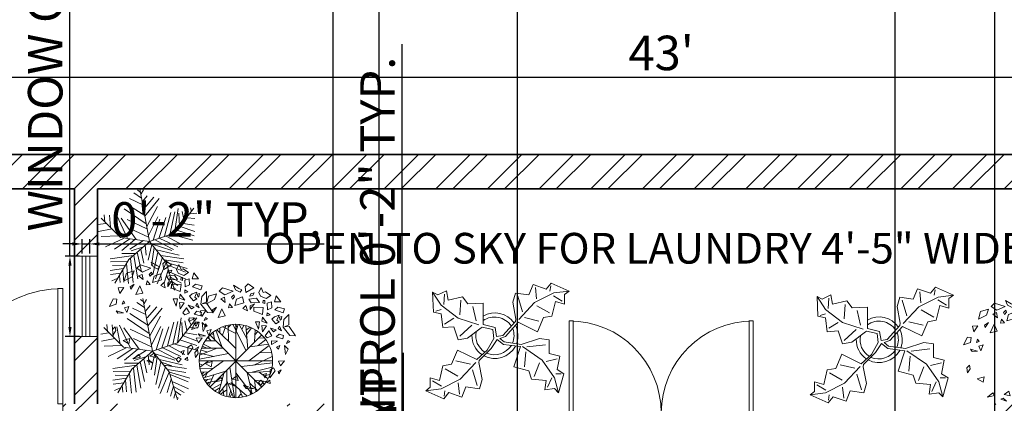
# Model space of a CAD drawing. Units: inches. Extents: x 744 to 1448, y 5126 to 6077.
# Tile 8 of 10: x 895 to 1152, y 5757 to 5857. Entities that reach past the tile are written whole.
import ezdxf

# ---------------------------------------------------------------- set-up
doc = ezdxf.new("R2010")
doc.units = ezdxf.units.IN
for name, color, linetype, lineweight in [('A-ANNO-DIMS', 2, 'Continuous', 18), ('A-AREA-IDEN', 7, 'Continuous', 18), ('A-DOOR', 4, 'Continuous', 18), ('A-WALL', 7, 'Continuous', 35), ('A-WALL-PATT', 252, 'Continuous', 13), ('L-PLNT', 3, 'Continuous', 13)]:
    doc.layers.add(name, color=color, linetype=linetype, lineweight=lineweight)
doc.layers.add('A-GLAZ', color=244, linetype='Continuous', lineweight=18, true_color=0x991b1e)
doc.styles.get("Standard").update_dxf_attribs({"font": 'arial.ttf'})
doc.dimstyles.new('ISO-25', dxfattribs={"dimtxt": 9, "dimasz": 2.5, "dimexe": 1.25, "dimexo": 0.625, "dimtad": 1, "dimlunit": 3, "dimtxsty": 'Standard', "dimcen": 2.5, "dimadec": 0, "dimazin": 0, "dimtfac": 1, "dimtmove": 0, "dimatfit": 3, "dimfxl": 1, "dimarcsym": 0})

# ---------------------------------------------------------------- blocks, each defined once
blk = doc.blocks.new('*U4')
for p, q in [((0, 0), (0, 6)), ((40, 0), (40, 6))]:
    blk.add_line(p, q)
blk.add_lwpolyline([(0, 0), (0, -40), (1.75, -40), (1.75, 0)], close=True)
blk.add_arc((0, 0), 40, 270, 0)
blk = doc.blocks.new('*U2')
for p, q in [((0, 0), (0, -6)), ((40, 0), (40, -6))]:
    blk.add_line(p, q)
blk.add_lwpolyline([(0, 0), (0, 40), (1.75, 40), (1.75, 0)], close=True)
blk.add_arc((0, 0), 40, 0, 90)
blk = doc.blocks.new('*U6')
for p, q in [((0, 0), (0, -6)), ((-40, 0), (-40, -6))]:
    blk.add_line(p, q)
blk.add_lwpolyline([(0, 0), (0, 40), (-1.75, 40), (-1.75, 0)], close=True)
blk.add_arc((0, 0), 40, 90, 180)
blk = doc.blocks.new('*U10')
for p, q in [((-10.186, 53.64), (-13.084, 55.962)), ((0, 0), (-10.5, 57)), ((-9.099, 51.782), (-6.563, 55.962)), ((-7.288, 39.707), (-21.778, 46.673)), ((-8.737, 47.138), (-17.069, 52.711)), ((-7.65, 43.423), (-2.578, 49.46)), ((-5.839, 35.992), (4.667, 48.067)), ((-5.114, 27.632), (10.463, 46.673)), ((-3.665, 19.273), (-27.574, 35.527)), ((-5.114, 28.097), (-24.676, 40.636)), ((-2.941, 16.486), (8.652, 37.85)), ((22.055, 7.198), (27.489, 32.277)), ((27, 9), (48, 36)), ((27.127, 9.056), (31.112, 35.992)), ((35.096, 32.741), (37.27, 22.524)), ((38.719, 34.134), (41.979, 28.561)), ((44.153, 36.456), (45.239, 32.741)), ((-31.5, 4.5), (-52.5, 25.5)), ((-48.585, 21.131), (-49.309, 29.026)), ((-43.513, 28.561), (-42.427, 15.558)), ((-38.442, 26.239), (-34.819, 7.663)), ((-35.544, 28.097), (-24.314, 3.947)), ((-14.533, 2.09), (-30.834, 25.31)), ((-24.314, 23.917), (-2.941, 13.7)), ((-1.129, 6.734), (9.014, 26.704)), ((3.942, 1.625), (11.187, 24.381)), ((10.101, 3.483), (17.708, 26.239)), ((16.259, 5.805), (23.142, 31.348)), ((31.836, 30.883), (32.561, 16.486)), ((40.53, 25.775), (48.862, 24.846)), ((43.791, 29.954), (51.036, 30.883)), ((-47.498, 19.737), (-55.83, 18.344)), ((-40.615, 13.7), (-55.105, 10.913)), ((-20.691, 13.7), (-1.129, 4.876)), ((29.662, 12.307), (48.137, 6.269)), ((33.285, 16.486), (48.862, 10.913)), ((36.183, 19.737), (48.137, 17.88)), ((-33.37, 6.269), (-52.207, 5.34)), ((-28.299, 3.483), (-47.86, -5.805)), ((-21.416, 3.018), (-38.079, -8.128)), ((0, 0), (-31.5, 4.5)), ((-15.982, 2.09), (-30.11, -9.521)), ((0, 0), (-22.5, -19.5)), ((-6.563, 1.161), (-21.416, -8.128)), ((0, 0), (27, 9)), ((0, 0), (18, -22.5)), ((6.478, 1.625), (26.04, -8.592)), ((11.187, 3.483), (30.749, -5.805)), ((18.07, 5.805), (35.096, -3.483)), ((24.229, 7.663), (46.688, 1.625)), ((-6.563, -5.805), (-19.967, -9.985)), ((-9.461, -8.592), (-6.201, -23.453)), ((-4.752, -3.483), (-3.665, -14.629)), ((2.493, -3.019), (-1.491, -20.202)), ((1.769, -2.555), (24.229, -9.521)), ((5.029, -6.27), (2.131, -25.775)), ((7.565, -9.056), (32.198, -14.629)), ((-17.431, -15.094), (-42.789, -18.809)), ((-22.5, -19.5), (-37.5, -45)), ((-15.257, -12.772), (-30.11, -12.772)), ((-20.691, -18.345), (-17.793, -44.352)), ((-17.069, -15.094), (-12.721, -40.172)), ((-13.446, -11.378), (-8.737, -32.741)), ((9.014, -11.378), (3.58, -35.992)), ((14.085, -16.951), (6.478, -40.172)), ((12.274, -15.094), (36.907, -18.809)), ((16.259, -19.738), (36.183, -22.989)), ((-28.299, -29.026), (-42.789, -31.348)), ((-24.314, -21.596), (-42.427, -22.06)), ((-26.849, -26.24), (-40.253, -25.775)), ((-29.023, -30.884), (-27.936, -43.887)), ((-25.038, -23.918), (-22.865, -45.281)), ((18.07, -22.524), (8.289, -45.745)), ((20.244, -30.419), (15.897, -44.816)), ((18, -22.5), (27, -52.5)), ((18.433, -22.524), (40.53, -29.026)), ((19.157, -25.311), (38.719, -33.206)), ((-30.834, -34.135), (-42.427, -35.528)), ((-34.457, -39.708), (-40.978, -42.494)), ((-32.646, -36.921), (-31.921, -44.352)), ((22.78, -37.85), (19.519, -48.532)), ((21.331, -32.741), (39.081, -40.636)), ((22.78, -38.314), (34.372, -44.816)), ((24.591, -45.745), (23.142, -50.854)), ((24.591, -43.423), (30.749, -47.603)), ((26.764, -49.925), (28.213, -50.854))]:
    blk.add_line(p, q)
blk = doc.blocks.new('*U11')
for points in [[(-4.43, 11.05), (-5.18, 10.36), (-3.96, 9.49), (-2.07, 10.36)], [(-2, 11.66), (-1.6, 10.62), (-0.52, 10.1), (-0.18, 10.62), (-0.79, 10.96)], [(1.24, 12), (0.56, 11.31), (0.76, 10.01), (2.52, 11.05)], [(4.14, 11.14), (3.6, 10.01), (4, 9.23), (5.22, 8.71), (6.3, 9.41), (5.08, 10.19), (4.61, 10.01)], [(-5.78, 9.75), (-7.54, 9.23), (-8.01, 7.5), (-6.26, 8.45)], [(-4.84, 8.63), (-3.83, 7.85), (-4.03, 8.97)], [(-1.94, 9.49), (-2.48, 8.97), (-2.27, 8.54), (-1.8, 9.06)], [(0.02, 9.06), (-1.33, 8.54), (-1.73, 7.16), (0.29, 7.76)], [(1.37, 8.54), (3.13, 8.8), (3.8, 7.85), (1.91, 7.76)], [(2.59, 9.93), (1.84, 9.75), (1.64, 9.23), (2.32, 9.41)], [(7.45, 9.32), (7.11, 7.94), (8.52, 7.94)], [(-5.78, 6.81), (-6.66, 6.21), (-6.52, 5.69)], [(-2.88, 7.5), (-3.15, 6.64), (-2.27, 6.72)], [(0.76, 7.16), (0.09, 6.46), (1.1, 5.95)], [(1.71, 6.29), (1.71, 7.07), (2.65, 7.5), (2.11, 6.9)], [(2.52, 6.81), (2.52, 5.86), (4.41, 5.17), (4.61, 6.72)], [(4.61, 8.28), (4.54, 7.76), (4.95, 7.59), (4.95, 8.28)], [(6.43, 7.94), (5.49, 7.68), (5.56, 6.21), (6.5, 6.64)], [(7.85, 6.81), (7.18, 6.21), (9, 5.51), (9.33, 6.38)], [(-8.14, 6.03), (-9.36, 5.95), (-9.02, 4.73)], [(-4.57, 6.38), (-5.45, 4.47), (-3.89, 4.82)], [(4.41, 4.56), (4.27, 3.7), (5.49, 3.26)], [(5.49, 5.51), (5.42, 4.82), (6.16, 5.08)], [(8.12, 4.99), (7.11, 4.65), (6.5, 4.13), (7.38, 3.09), (8.12, 3.52), (7.65, 3.87)], [(8.73, 4.73), (8.19, 4.56), (8.39, 3.87), (8.59, 4.04)], [(10.28, 5.17), (9.2, 4.04), (9, 2.31), (10.48, 0.49), (11.76, 0.41), (10.35, 2.48), (9.33, 2.4), (10.28, 2.83)], [(-11.32, 1.79), (-9.83, 2.31), (-9.63, 3.44), (-10.44, 3.52)], [(-8.21, 3.09), (-8.48, 2.31), (-7.87, 2.57)], [(3.53, 1.88), (2.86, 3.52), (3.8, 3.52)], [(4.27, 2.74), (5.29, 2.66), (4.41, 1.27)], [(8.19, 2.57), (7.92, 2.05), (8.66, 1.53)], [(-8.21, 0.41), (-9.43, 0.32), (-9.83, 0.84)], [(-7, 1.79), (-7.94, 1.53), (-7.47, 0.49)], [(5.83, 1.53), (5.02, 0.41), (5.49, -0.02), (6.5, 0.41)], [(7.51, 1.71), (6.91, 1.27), (6.23, 2.14)], [(8.12, 0.75), (7.51, 0.15), (8.93, -0.28), (9.13, 0.49)], [(7.78, -0.8), (6.43, -1.5), (6.43, -0.72)], [(8.32, -1.75), (7.98, -2.53), (7.58, -2.1)], [(9.33, -1.75), (9.54, -3.74), (10.14, -2.53)], [(10.08, -0.63), (9.74, -1.32), (10.48, -0.89)], [(-10.03, -2.71), (-10.64, -3.31), (-10.44, -4.44), (-9.9, -3.49)], [(-8.28, -5.73), (-6.79, -5.3), (-7, -6.51)], [(9.33, -5.13), (8.46, -6.25), (7.98, -5.22)], [(-2.34, -9.2), (-1.26, -8.5), (-0.99, -9.54)], [(5.29, -7.98), (4.61, -8.16), (5.02, -8.94)], [(6.1, -8.94), (6.16, -7.21), (6.91, -6.69), (7.24, -7.38)], [(8.05, -8.07), (8.59, -7.12), (7.92, -7.55)], [(-4.84, -8.85), (-4.43, -9.45), (-5.99, -9.8)], [(-2.54, -10.06), (-3.02, -10.23), (-1.8, -10.67)], [(0.22, -10.58), (0.83, -11.27), (2.59, -11.36)], [(4.07, -9.45), (3.53, -9.97), (4.07, -10.58), (4.61, -9.89)], [(6.03, -9.45), (5.42, -9.97), (6.16, -10.15)]]:
    blk.add_lwpolyline(points, close=True)
blk = doc.blocks.new('Plant - Rubber or Philodendron')
for p, q in [((8.8871, 10.7908), (9.9809, 13.4933)), ((9.9809, 13.4933), (13.3837, 12.301)), ((13.3837, 12.301), (14.68, 13.9039)), ((14.5816, 13.2037), (14.3848, 11.8033)), ((14.68, 13.9039), (19.3848, 11.8146)), ((-16.2005, 11.4774), (-13.9899, 8.1064)), ((-16.2005, 11.4774), (-14.8639, 10.7964)), ((-16.0159, 6.3329), (-16.2005, 11.4774)), ((-14.8639, 10.7964), (-12.6195, 11.8975)), ((-13.3174, 8.325), (-13.0735, 11.0065)), ((-12.6195, 11.8975), (-12.1909, 9.4345)), ((-12.1909, 9.4345), (-8.3829, 10.3)), ((-8.3829, 10.3), (-7.0549, 8.501)), ((4.6914, 8.8812), (5.3859, 11.2828)), ((5.3859, 11.2828), (8.8871, 10.7908)), ((5.9878, 10.4842), (7.1971, 6.3869)), ((15.3859, 11.3055), (10.3916, 8.7942)), ((10.5828, 12.6946), (10.8893, 9.7953)), ((15.2875, 10.6053), (17.5907, 9.2105)), ((19.3848, 11.8146), (15.3859, 11.3055)), ((19.3848, 11.8146), (18.1868, 10.9119)), ((18.1868, 10.9119), (18.1925, 8.4119)), ((-13.9899, 8.1064), (-9.5434, 4.7185)), ((-8.8369, 9.409), (-9.0894, 5.6095)), ((-7.0549, 8.501), (-3.0284, 8.6941)), ((-4.8529, 4.012), (-5.7184, 7.82)), ((-3.0284, 8.6941), (-3.0709, 3.1041)), ((4.6914, 8.8812), (5.5014, 4.4831)), ((10.3916, 8.7942), (6.2847, 4.4028)), ((14.2977, 6.1031), (10.9934, 7.9956)), ((15.7909, 9.1065), (14.8995, 5.3044)), ((18.1925, 8.4119), (15.7909, 9.1065)), ((-14.0069, 5.8704), (-16.0159, 6.3329)), ((-15.3434, 6.5514), (-13.9984, 6.9884)), ((-13.5868, 2.2894), (-14.0069, 5.8704)), ((14.8995, 5.3044), (12.7005, 4.8994)), ((-13.1329, 3.1804), (-10.6614, 4.727)), ((-9.5434, 4.7185), (-4.1917, 2.9888)), ((-9.1318, 0.0195), (-5.9793, 2.9025)), ((-3.0709, 3.1041), (0.0797, 2.3163)), ((2.1141, 0.2298), (5.4346, 3.9146)), ((6.1032, 3.6844), (2.8262, -0.031)), ((5.4346, 3.9146), (5.5014, 4.4831)), ((11.1089, 1.1958), (6.1032, 3.6844)), ((7.7005, 4.8881), (11.5025, 3.9967)), ((12.7005, 4.8994), (11.1089, 1.1958)), ((-10.6784, 2.491), (-13.5868, 2.2894)), ((-9.5858, -0.8715), (-10.6784, 2.491)), ((-7.1228, -0.443), (-3.5248, 2.2131)), ((-3.5248, 2.2131), (-3.3011, 2.4355)), ((-3.3011, 2.4355), (-0.5306, 1.7947)), ((-0.5306, 1.7947), (-0.2255, -0.5527)), ((-0.5306, 1.7947), (-0.5306, 1.7947)), ((0.0797, 2.3163), (0.4866, -0.031)), ((0.4866, -0.031), (2.1141, 0.2298)), ((-7.1228, -0.443), (-9.5858, -0.8715)), ((-2.019, -3.6148), (-0.2255, -0.5527)), ((-0.9375, -3.1608), (0.5883, -0.8135)), ((0.5883, -0.8135), (2.2447, -2.0916)), ((2.8262, -0.031), (1.3003, -0.5527)), ((1.3003, -0.5527), (2.4193, -1.4655)), ((2.2447, -2.0916), (6.7108, -2.6626)), ((2.4193, -1.4655), (6.895, -2.1175)), ((11.6605, -0.5413), (6.895, -2.1175)), ((8.3544, -2.7453), (13.1973, -2.1704)), ((11.6605, -0.5413), (14.1354, -0.8948)), ((14.1354, -0.8948), (14.1354, -4.4304)), ((-11.3237, -7.2629), (-9.7321, -3.5593)), ((-9.7321, -3.5593), (-4.7264, -6.0479)), ((-2.019, -3.6148), (-4.7264, -6.0479)), ((-4.0579, -6.2781), (-0.9375, -3.1608)), ((4.943, -7.9659), (6.7108, -2.6626)), ((12.3677, -6.1981), (7.219, -2.6772)), ((8.125, -4.0768), (7.7715, -7.9659)), ((14.1354, -4.4304), (16.9638, -5.1375)), ((-14.4141, -11.4699), (-13.5228, -7.6679)), ((-13.5228, -7.6679), (-11.3237, -7.2629)), ((-6.3237, -7.2516), (-10.1257, -6.3602)), ((-9.0148, -11.1577), (-4.9047, -6.8122)), ((-4.1246, -6.8466), (-4.0579, -6.2781)), ((-3.3146, -11.2447), (-4.1246, -6.8466)), ((10.2463, -10.4408), (11.6605, -6.9053)), ((15.5496, -10.7943), (12.3677, -6.1981)), ((16.2567, -5.8446), (13.4283, -6.5517)), ((16.9638, -5.1375), (16.2567, -8.673)), ((-12.921, -8.4665), (-9.6166, -10.359)), ((-4.611, -12.8477), (-5.8203, -8.7504)), ((8.8321, -9.0266), (4.943, -7.9659)), ((9.5392, -11.1479), (8.8321, -9.0266)), ((17.3174, -9.7337), (15.9032, -9.7337)), ((16.2567, -8.673), (18.0245, -9.7337)), ((18.0245, -9.7337), (16.6103, -14.6834)), ((-16.8157, -10.7754), (-14.4141, -11.4699)), ((-16.8101, -13.2754), (-16.8157, -10.7754)), ((-13.9107, -12.9688), (-16.2139, -11.574)), ((-14.0091, -13.669), (-9.0148, -11.1577)), ((-9.206, -15.0581), (-9.5126, -12.1588)), ((-3.3146, -11.2447), (-4.0092, -13.6463)), ((13.4283, -11.5015), (9.5392, -11.1479)), ((13.0748, -13.9763), (13.4283, -11.5015)), ((14.8425, -10.7943), (13.7819, -13.2692)), ((16.6103, -14.6834), (15.5496, -10.7943)), ((-18.008, -14.1781), (-16.8101, -13.2754)), ((-18.008, -14.1781), (-14.0091, -13.669)), ((-13.3032, -16.2674), (-18.008, -14.1781)), ((-12.0069, -14.6645), (-13.3032, -16.2674)), ((-13.2048, -15.5672), (-13.008, -14.1668)), ((-8.6042, -15.8568), (-12.0069, -14.6645)), ((-7.5103, -13.1543), (-8.6042, -15.8568)), ((-4.0092, -13.6463), (-7.5103, -13.1543)), ((15.5496, -13.6228), (13.0748, -13.9763)), ((16.6103, -14.6834), (15.5496, -13.6228))]:
    blk.add_line(p, q)
for centre, radius, start, end in [((0, 0), 6.1275, 34.37569, 120.1028), ((-0.0601, -0.2075), 5.2461, 33.82192, 124.9414), ((-0.098, 0.1364), 6.1288, 341.2017, 26.09184), ((0.0308, 0.1664), 6, 178.6147, 235.1169), ((0.0308, 0.1664), 5, 168.1647, 238.6725), ((-0.2664, 0.1682), 5.2775, 338.4094, 20.03007), ((-0.1102, 0.4886), 5.2883, 247.3711, 327.472), ((-0.0234, 0.3825), 6.1492, 242.5812, 331.2714)]:
    blk.add_arc(centre, radius, start, end)
blk = doc.blocks.new('*U13')
for p, q in [((-32.6092, 50.4264), (-23.2782, 23.5674)), ((-31.2008, 51.1035), (-0.2149, 20.1818)), ((-26.4472, 46.5894), (-26.2712, 53.8116)), ((-22.0458, 42.0753), (-16.5881, 57.6486)), ((-21.1656, 55.8436), (-0.0388, 45.0094)), ((-12.5388, 54.9406), (-7.9613, 59.4546)), ((-12.3627, 32.1443), (-12.5388, 58.7776)), ((-5.3205, 59.6806), (16.5105, 16.7963)), ((2.426, 54.9406), (-1.4472, 59.9056)), ((0, 59.9996), (0, -60)), ((0.4894, 48.6208), (3.6584, 59.6806)), ((18.2711, 35.5298), (5.419, 59.6806)), ((9.8203, 51.5549), (12.8133, 58.5516)), ((19.6795, 19.5047), (16.3344, 57.6486)), ((17.0387, 51.1035), (23.2006, 55.1666)), ((17.7429, 43.6552), (25.4894, 54.2636)), ((31.6513, 50.8778), (30.2429, 30.5643)), ((-49.8627, 32.8214), (-32.7853, 32.8214)), ((-45.8134, 38.2383), (-40.5318, 33.0471)), ((-43.8768, 36.4326), (-44.405, 40.2696)), ((42, 42), (-42, -42)), ((42, -42), (-42, 42)), ((-40.1797, 44.558), (-36.4825, 43.2038)), ((-37.0107, 47.0408), (-35.25, 35.5298)), ((31.1232, 42.5267), (35.8767, 48.1693)), ((36.2288, 25.1474), (48.9049, 35.0784)), ((37.1091, 37.1098), (46.6161, 37.5612)), ((-32.2571, 20.6333), (-59.1937, 9.348)), ((-57.081, 17.9248), (-47.0458, 14.7649)), ((-56.0247, 20.859), (-20.8134, 20.859)), ((-54.7923, 24.4702), (-47.75, 21.0847)), ((-53.2078, 27.4044), (-40.1797, 20.859)), ((54.3626, 25.3731), (20.9119, 0.3198)), ((23.3767, 23.3417), (53.3063, 27.4044)), ((-59.7219, 2.8025), (-12.0106, 12.0565)), ((-58.6656, 12.7336), (-35.9543, 7.5424)), ((-54.6162, -24.7335), (-20.2853, 0.0941)), ((29.3626, -6.6771), (59.4682, 7.091)), ((38.5175, 13.4107), (58.2359, 13.6364)), ((-60, 0), (60, 0)), ((-59.7219, -4.8714), (-54.2641, -6.6771)), ((-45.2853, -0.1316), (-59.0177, -10.0627)), ((-58.4895, -12.3197), (-36.4825, -11.6426)), ((-14.8275, -15.0282), (-14.6515, -57.6865)), ((-10.074, -10.0627), (-2.5036, -59.7178)), ((9.2922, -9.1598), (59.6443, -2.8401)), ((26.3697, -18.4138), (58.9401, -9.8369)), ((-57.081, -18.4138), (-45.2853, -17.9624)), ((-52.6797, -18.188), (-55.4966, -22.0251)), ((-53.2078, -27.442), (-16.7641, -16.6081)), ((-38.9472, -29.0219), (-51.4472, -30.6018)), ((-47.2219, -19.3166), (-50.2148, -26.3135)), ((-46.5177, -30.1504), (-49.5106, -33.536)), ((-35.9543, -22.4765), (-44.0529, -40.5329)), ((-19.9331, -20.2194), (-28.5599, -52.721)), ((-0.0388, -19.0909), (25.8415, -53.8495)), ((18.6232, -18.6394), (26.7218, -53.3981)), ((18.7992, -18.6394), (57.3556, -17.2853)), ((30.419, -30.1504), (32.3556, -50.0125)), ((31.4753, -31.279), (49.6091, -33.3103)), ((38.1654, -18.188), (52.426, -29.0219)), ((45.9119, -24.0564), (55.595, -22.2508)), ((-32.4331, -32.4075), (-48.1021, -35.5674)), ((-43.7008, -34.6645), (-46.6937, -37.373)), ((-24.6867, -37.8244), (-38.7712, -45.7241)), ((-26.2712, -43.9185), (-34.7219, -48.6583)), ((-14.6515, -36.2445), (-27.6797, -52.9467)), ((-14.6515, -47.3041), (-25.0388, -54.3009)), ((-21.5177, -45.4984), (-19.9331, -56.1065)), ((-14.6515, -32.1818), (-3.912, -59.4922)), ((-8.4895, -47.5298), (-11.4825, -58.5893)), ((-6.2008, -36.2445), (17.919, -57.0094)), ((5.9471, -46.6269), (10.5246, -58.5893)), ((22.8485, -36.4702), (35.3485, -48.4326)), ((24.7852, -44.8213), (23.0246, -54.978)), ((41.5105, -32.6332), (46.088, -38.0501)), ((-6.3768, -52.721), (-9.3698, -58.815)), ((8.4119, -53.1724), (3.8344, -59.4922))]:
    blk.add_line(p, q)
blk.add_circle((0, 0), 60)
blk = doc.blocks.new('*D24')
at = {"layer": 'A-ANNO-DIMS', "color": 0, "lineweight": -2, "transparency": 16777216}
for p, q in [((804.68, 5822.44), (804.68, 5843.13)), ((1320.68, 5822.44), (1320.68, 5843.13)), ((1318.18, 5841.88), (807.18, 5841.88))]:
    blk.add_line(p, q, dxfattribs=at)
at = {"layer": 'A-ANNO-DIMS', "color": 0, "transparency": 16777216}
for points in [[(807.18, 5842.3), (807.18, 5841.46), (804.68, 5841.88)], [(1318.18, 5842.3), (1318.18, 5841.46), (1320.68, 5841.88)]]:
    blk.add_solid(points, dxfattribs=at)
at = {"layer": 'Defpoints', "color": 0, "transparency": 16777216}
for p in [(804.68, 5841.88), (804.68, 5821.82), (1320.68, 5821.82)]:
    blk.add_point(p, dxfattribs=at)
at = {"layer": 'A-ANNO-DIMS', "color": 0, "transparency": 16777216, "insert": (1062.68, 5847.1), "char_height": 9, "attachment_point": 5}
blk.add_mtext("43'", dxfattribs=at)
blk = doc.blocks.new('WINDOW-GLASS-21IN')
for p, q in [((0, 21), (0, 0)), ((1, 21), (1, 0)), ((2, 21), (2, 0))]:
    blk.add_line(p, q)
blk = doc.blocks.new('*D41')
at = {"layer": 'A-ANNO-DIMS', "color": 0, "lineweight": -2, "transparency": 16777216}
for p, q in [((908.53, 5795.32), (908.53, 5925.53)), ((911.06, 5795.32), (907.28, 5795.32)), ((908.53, 5776.82), (908.53, 5792.82)), ((911.06, 5774.32), (907.28, 5774.32))]:
    blk.add_line(p, q, dxfattribs=at)
at = {"layer": 'A-ANNO-DIMS', "color": 0, "transparency": 16777216}
for points in [[(908.12, 5792.82), (908.95, 5792.82), (908.53, 5795.32)], [(908.12, 5776.82), (908.95, 5776.82), (908.53, 5774.32)]]:
    blk.add_solid(points, dxfattribs=at)
at = {"layer": 'Defpoints', "color": 0, "transparency": 16777216}
for p in [(908.53, 5795.32), (911.68, 5795.32), (911.68, 5774.32)]:
    blk.add_point(p, dxfattribs=at)
at = {"layer": 'A-ANNO-DIMS', "color": 0, "transparency": 16777216, "insert": (903.25, 5861.67), "char_height": 9, "attachment_point": 5, "rotation": 90}
blk.add_mtext('WINDOW C 1\'-9" TYP.', dxfattribs=at)
blk = doc.blocks.new('*D42')
at = {"layer": 'A-ANNO-DIMS', "color": 0, "lineweight": -2, "transparency": 16777216}
for p, q in [((911.68, 5795.94), (911.68, 5799.72)), ((913.68, 5795.94), (913.68, 5799.72)), ((909.18, 5798.47), (906.68, 5798.47)), ((911.68, 5798.47), (913.68, 5798.47)), ((916.18, 5798.47), (974.79, 5798.47))]:
    blk.add_line(p, q, dxfattribs=at)
at = {"layer": 'A-ANNO-DIMS', "color": 0, "transparency": 16777216}
for points in [[(909.18, 5798.88), (909.18, 5798.05), (911.68, 5798.47)], [(916.18, 5798.88), (916.18, 5798.05), (913.68, 5798.47)]]:
    blk.add_solid(points, dxfattribs=at)
at = {"layer": 'Defpoints', "color": 0, "transparency": 16777216}
for p in [(913.68, 5798.47), (911.68, 5795.32), (913.68, 5795.32)]:
    blk.add_point(p, dxfattribs=at)
at = {"layer": 'A-ANNO-DIMS', "color": 0, "transparency": 16777216, "insert": (946.74, 5803.69), "char_height": 9, "attachment_point": 5}
blk.add_mtext('0\'-2" TYP.', dxfattribs=at)
blk = doc.blocks.new('*D50')
at = {"layer": 'A-ANNO-DIMS', "color": 0, "lineweight": -2, "transparency": 16777216}
for p, q in [((995.52, 5712.29), (995.52, 5770.05)), ((994.35, 5712.29), (996.77, 5712.29)), ((995.52, 5702.85), (995.52, 5709.79)), ((994.35, 5700.35), (996.77, 5700.35))]:
    blk.add_line(p, q, dxfattribs=at)
at = {"layer": 'A-ANNO-DIMS', "color": 0, "transparency": 16777216}
for points in [[(995.1, 5709.79), (995.93, 5709.79), (995.52, 5712.29)], [(995.1, 5702.85), (995.93, 5702.85), (995.52, 5700.35)]]:
    blk.add_solid(points, dxfattribs=at)
at = {"layer": 'Defpoints', "color": 0, "transparency": 16777216}
for p in [(993.72, 5712.29), (995.52, 5712.29), (993.72, 5700.35)]:
    blk.add_point(p, dxfattribs=at)
at = {"layer": 'A-ANNO-DIMS', "color": 0, "transparency": 16777216, "insert": (990.3, 5742.42), "char_height": 9, "attachment_point": 5, "rotation": 90}
blk.add_mtext('1\'-0" TYP.', dxfattribs=at)
blk = doc.blocks.new('*D51')
at = {"layer": 'A-ANNO-DIMS', "color": 0, "lineweight": -2, "transparency": 16777216}
for p, q in [((995.17, 5727.09), (995.17, 5850.56)), ((994.84, 5724.59), (993.92, 5724.59)), ((994.84, 5722.64), (993.92, 5722.64)), ((995.17, 5722.64), (995.17, 5724.59)), ((995.17, 5720.14), (995.17, 5717.64))]:
    blk.add_line(p, q, dxfattribs=at)
at = {"layer": 'A-ANNO-DIMS', "color": 0, "transparency": 16777216}
for points in [[(994.75, 5727.09), (995.58, 5727.09), (995.17, 5724.59)], [(994.75, 5720.14), (995.58, 5720.14), (995.17, 5722.64)]]:
    blk.add_solid(points, dxfattribs=at)
at = {"layer": 'Defpoints', "color": 0, "transparency": 16777216}
for p in [(995.17, 5724.59), (995.46, 5724.59), (995.46, 5722.64)]:
    blk.add_point(p, dxfattribs=at)
at = {"layer": 'A-ANNO-DIMS', "color": 0, "transparency": 16777216, "insert": (989.89, 5790.08), "char_height": 9, "attachment_point": 5, "rotation": 90}
blk.add_mtext('CONTROL 0\'-2" TYP.', dxfattribs=at)
blk = doc.blocks.new('*D55')
at = {"layer": 'A-ANNO-DIMS', "color": 0, "lineweight": -2, "transparency": 16777216}
for p, q in [((989.18, 5323.94), (989.18, 6059.61)), ((1025.18, 5323.94), (1025.18, 6059.61)), ((991.68, 6058.36), (1022.68, 6058.36))]:
    blk.add_line(p, q, dxfattribs=at)
at = {"layer": 'A-ANNO-DIMS', "color": 0, "transparency": 16777216}
for points in [[(991.68, 6058.78), (991.68, 6057.95), (989.18, 6058.36)], [(1022.68, 6058.78), (1022.68, 6057.95), (1025.18, 6058.36)]]:
    blk.add_solid(points, dxfattribs=at)
at = {"layer": 'Defpoints', "color": 0, "transparency": 16777216}
for p in [(1025.18, 6058.36), (989.18, 5323.32), (1025.18, 5323.32)]:
    blk.add_point(p, dxfattribs=at)
at = {"layer": 'A-ANNO-DIMS', "color": 0, "transparency": 16777216, "insert": (1007.18, 6063.59), "char_height": 9, "attachment_point": 5}
blk.add_mtext('3\'-0"', dxfattribs=at)
blk = doc.blocks.new('*D57')
at = {"layer": 'A-ANNO-DIMS', "color": 0, "lineweight": -2, "transparency": 16777216}
for p, q in [((1123.68, 5672.44), (1123.68, 6059.61)), ((1149.68, 5672.44), (1149.68, 6059.61)), ((1126.18, 6058.36), (1147.18, 6058.36))]:
    blk.add_line(p, q, dxfattribs=at)
at = {"layer": 'A-ANNO-DIMS', "color": 0, "transparency": 16777216}
for points in [[(1126.18, 6058.78), (1126.18, 6057.95), (1123.68, 6058.36)], [(1147.18, 6058.78), (1147.18, 6057.95), (1149.68, 6058.36)]]:
    blk.add_solid(points, dxfattribs=at)
at = {"layer": 'Defpoints', "color": 0, "transparency": 16777216}
for p in [(1149.68, 6058.36), (1123.68, 5671.82), (1149.68, 5671.82)]:
    blk.add_point(p, dxfattribs=at)
at = {"layer": 'A-ANNO-DIMS', "color": 0, "transparency": 16777216, "insert": (1136.68, 6063.51), "char_height": 9, "attachment_point": 5}
blk.add_mtext('2\'-2"', dxfattribs=at)
blk = doc.blocks.new('*D59')
at = {"layer": 'A-ANNO-DIMS', "color": 0, "lineweight": -2, "transparency": 16777216}
for p, q in [((762.28, 5746.58), (762.28, 5795.38)), ((1128.24, 5746.58), (761.03, 5746.58)), ((762.28, 5717.4), (762.28, 5744.08)), ((1128.24, 5714.9), (761.03, 5714.9))]:
    blk.add_line(p, q, dxfattribs=at)
at = {"layer": 'A-ANNO-DIMS', "color": 0, "transparency": 16777216}
for points in [[(761.87, 5744.08), (762.7, 5744.08), (762.28, 5746.58)], [(761.87, 5717.4), (762.7, 5717.4), (762.28, 5714.9)]]:
    blk.add_solid(points, dxfattribs=at)
at = {"layer": 'Defpoints', "color": 0, "transparency": 16777216}
for p in [(762.28, 5746.58), (1128.86, 5746.58), (1128.86, 5714.9)]:
    blk.add_point(p, dxfattribs=at)
at = {"layer": 'A-ANNO-DIMS', "color": 0, "transparency": 16777216, "insert": (757.01, 5772.23), "char_height": 9, "attachment_point": 5, "rotation": 90}
blk.add_mtext('2\'-7 1/2"', dxfattribs=at)
blk = doc.blocks.new('*D62')
at = {"layer": 'A-ANNO-DIMS', "color": 0, "lineweight": -2, "transparency": 16777216}
for p, q in [((816.68, 5262.94), (816.68, 6059.61)), ((977.18, 5262.94), (977.18, 6059.61)), ((819.18, 6058.36), (974.68, 6058.36))]:
    blk.add_line(p, q, dxfattribs=at)
at = {"layer": 'A-ANNO-DIMS', "color": 0, "transparency": 16777216}
for points in [[(819.18, 6058.78), (819.18, 6057.95), (816.68, 6058.36)], [(974.68, 6058.78), (974.68, 6057.95), (977.18, 6058.36)]]:
    blk.add_solid(points, dxfattribs=at)
at = {"layer": 'Defpoints', "color": 0, "transparency": 16777216}
for p in [(977.18, 6058.36), (816.68, 5262.32), (977.18, 5262.32)]:
    blk.add_point(p, dxfattribs=at)
at = {"layer": 'A-ANNO-DIMS', "color": 0, "transparency": 16777216, "insert": (896.93, 6063.64), "char_height": 9, "attachment_point": 5}
blk.add_mtext('13\'-4 1/2"', dxfattribs=at)

msp = doc.modelspace()

# ---------------------------------------------------------------- hatches: boundary and pattern name
at = {"layer": 'A-WALL-PATT'}
h = msp.add_hatch(dxfattribs=at)
h.set_pattern_fill('ANSI32', color=256)
h.paths.add_polyline_path([(813.684, 5750.816), (876.684, 5750.816), (876.684, 5756.816), (813.684, 5756.816), (813.684, 5812.816), (909.684, 5812.816), (909.684, 5795.316), (915.684, 5795.316), (915.684, 5812.816), (1209.684, 5812.816), (1209.684, 5795.316), (1215.684, 5795.316), (1215.684, 5812.816), (1311.684, 5812.816), (1311.684, 5756.816), (1248.684, 5756.816), (1248.684, 5750.816), (1311.684, 5750.816), (1311.684, 5570.816), (1179.044, 5570.816), (1179.044, 5564.816), (1311.684, 5564.816), (1311.684, 5383.316), (1260.684, 5383.316), (1260.684, 5377.316), (1311.684, 5377.316), (1311.684, 5320.316), (1227.684, 5320.316), (1227.684, 5333.816), (1221.684, 5333.816), (1221.684, 5314.316), (1320.684, 5314.316), (1320.684, 5821.816), (804.684, 5821.816), (804.684, 5472.316), (926.184, 5472.316), (926.184, 5481.316), (813.684, 5481.316), (813.684, 5581.616), (946.284, 5581.616), (946.284, 5587.616), (813.684, 5587.616)])
h.paths.add_polyline_path([(1155.684, 5525.816), (1149.684, 5525.816), (1149.684, 5481.316), (1025.184, 5481.316), (1025.184, 5475.316), (1146.684, 5475.316), (1146.684, 5323.316), (1118.788, 5323.316), (1118.788, 5314.316), (1146.684, 5314.316), (1155.684, 5314.316), (1155.684, 5374.316), (1170.35, 5374.316), (1170.35, 5383.316), (1155.684, 5383.316)], flags=17)
h.paths.add_polyline_path([(1230.684, 5383.316), (1213.35, 5383.316), (1213.35, 5374.316), (1221.684, 5374.316), (1221.684, 5363.816), (1226.184, 5363.816), (1227.684, 5363.816), (1227.684, 5377.316), (1230.684, 5377.316)], flags=17)
h.paths.add_polyline_path([(1185.684, 5671.816), (1155.684, 5671.816), (1155.684, 5750.816), (1161.575, 5750.816), (1161.575, 5756.816), (1157.542, 5756.816), (1157.847, 5756.715), (1155.79, 5756.816), (1149.684, 5756.816), (1149.684, 5750.816), (1149.684, 5671.816), (1121.684, 5671.816), (1121.684, 5665.816), (1179.684, 5665.816), (1179.684, 5609.816), (1185.684, 5609.816)], flags=17)
h.paths.add_polyline_path([(1003.684, 5671.816), (975.684, 5671.816), (975.684, 5750.816), (975.684, 5756.816), (965.205, 5756.816), (965.205, 5750.816), (969.684, 5750.816), (969.684, 5671.816), (939.684, 5671.816), (939.684, 5626.616), (945.684, 5626.616), (945.684, 5665.816), (1003.684, 5665.816)], flags=17)
h.paths.add_polyline_path([(915.684, 5774.316), (909.684, 5774.316), (909.684, 5756.816), (906.684, 5756.816), (906.684, 5752.316), (906.684, 5750.816), (922.205, 5750.816), (922.205, 5756.816), (915.684, 5756.816)], flags=17)
h.paths.add_polyline_path([(1215.684, 5774.316), (1209.684, 5774.316), (1209.684, 5756.816), (1204.575, 5756.816), (1204.575, 5750.816), (1218.684, 5750.816), (1218.684, 5756.816), (1215.684, 5756.816)], flags=17)
h.paths.add_polyline_path([(1063.788, 5323.316), (1025.184, 5323.316), (1025.184, 5314.316), (1063.788, 5314.316)])
h.paths.add_polyline_path([(986.184, 5475.316), (989.184, 5475.316), (989.184, 5481.316), (974.184, 5481.316), (974.184, 5475.916), (974.184, 5472.316), (977.184, 5472.316), (977.184, 5314.316), (989.184, 5314.316), (989.184, 5319.716), (989.184, 5323.316), (986.184, 5323.316)])

# ---------------------------------------------------------------- linework, layer by layer
at = {"layer": 'A-GLAZ'}
msp.add_lwpolyline([(909.684, 5795.316), (915.684, 5795.316), (915.684, 5774.316), (909.684, 5774.316)], close=True, dxfattribs=at)
at = {"layer": 'A-WALL'}
for p, q in [((804.684, 5821.816), (1320.684, 5821.816)), ((813.684, 5812.816), (909.684, 5812.816)), ((909.684, 5756.816), (909.684, 5812.816)), ((915.684, 5756.816), (915.684, 5812.816)), ((915.684, 5812.816), (1209.684, 5812.816))]:
    msp.add_line(p, q, dxfattribs=at)

# ---------------------------------------------------------------- block references
at = {"layer": 'A-DOOR', "xscale": 0.75, "yscale": 0.75, "zscale": 0.75, "rotation": 180.0000000000004}
msp.add_blockref('*U4', (906.684, 5756.816), dxfattribs=at)
at = {"layer": 'A-DOOR', "xscale": 0.6, "yscale": 0.6, "zscale": 0.6}
for name, p in [('*U2', (1038.684, 5754.416)), ('*U6', (1086.684, 5754.416))]:
    msp.add_blockref(name, p, dxfattribs=at)
at = {"layer": 'A-GLAZ'}
msp.add_blockref('WINDOW-GLASS-21IN', (911.684, 5774.316), dxfattribs=at)
at = {"layer": 'L-PLNT'}
for name, p, xscale, yscale, zscale in [('*U10', (929.291, 5799.083), 0.2409161369388113, 0.2409161369388113, 0.2409161369388113), ('*U11', (932.084, 5780.026), 1.172842970614158, 1.172842970614158, 1.172842970614158), ('*U11', (953.532, 5774.036), 1.172842970614158, 1.172842970614158, 1.172842970614158), ('*U10', (930.049, 5770.508), 0.2409161369388113, 0.2409161369388113, 0.2409161369388113), ('*U11', (1154.815, 5770.036), 1.172842970614158, 1.172842970614158, 1.172842970614158), ('*U13', (951.806, 5767.957), 0.1595845373812122, 0.1595845373812122, 0.1595845373812122)]:
    msp.add_blockref(name, p, dxfattribs=dict(at, xscale=xscale, yscale=yscale, zscale=zscale))
for p in [(1019.299, 5774.379), (1119.505, 5773.302)]:
    msp.add_blockref('Plant - Rubber or Philodendron', p, dxfattribs=at)

# ---------------------------------------------------------------- texts
at = {"layer": 'A-AREA-IDEN', "insert": (959.254, 5801.351), "char_height": 8, "attachment_point": 1}
msp.add_mtext_dynamic_manual_height_columns('OPEN TO SKY FOR LAUNDRY 4\'-5" WIDE', width=218.47208, gutter_width=12.5, heights=[0], dxfattribs=at)

# ---------------------------------------------------------------- dimensions: what is measured, and where the dimension line sits
at = {"layer": 'A-ANNO-DIMS'}
for base, p1, p2, override, picture, middle in [((977.184, 6058.363), (816.684, 5262.316), (977.184, 5262.316), {"dimdec": 1, "dimlfac": 1, "dimrnd": 0, "dimzin": 1, "dimdsep": 46, "dimlunit": 4, "dimfrac": 2}, '*D62', (896.934, 6063.645)), ((1025.184, 6058.363), (989.184, 5323.316), (1025.184, 5323.316), {"dimdec": 1, "dimlfac": 1, "dimrnd": 0, "dimzin": 1, "dimdsep": 46, "dimlunit": 4, "dimfrac": 2}, '*D55', (1007.184, 6063.586)), ((1149.684, 6058.363), (1123.684, 5671.816), (1149.684, 5671.816), {"dimdec": 1, "dimlfac": 1, "dimrnd": 0, "dimzin": 1, "dimdsep": 46, "dimlunit": 4, "dimfrac": 2}, '*D57', (1136.684, 6063.507)), ((804.684, 5841.882), (1320.684, 5821.816), (804.684, 5821.816), {"dimclrd": 0, "dimclre": 0, "dimclrt": 0}, '*D24', (1062.684, 5847.105))]:
    dim = msp.add_linear_dim(base=base, p1=p1, p2=p2, dimstyle='ISO-25', override=override, dxfattribs=at)
    dim.commit()
    dim.dimension.update_dxf_attribs({"geometry": picture, "text_midpoint": middle})
for base, p1, p2, text, picture, middle in [((908.534, 5795.316), (911.684, 5774.316), (911.684, 5795.316), 'WINDOW C <> TYP.', '*D41', (903.253, 5861.671)), ((995.168, 5724.594), (995.462, 5722.636), (995.462, 5724.594), 'CONTROL <> TYP.', '*D51', (989.886, 5790.079)), ((995.516, 5712.288), (993.724, 5700.346), (993.724, 5712.288), '<> TYP.', '*D50', (990.296, 5742.42))]:
    dim = msp.add_linear_dim(base=base, p1=p1, p2=p2, angle=90, text=text, dimstyle='ISO-25', override={"dimdec": 1, "dimlfac": 1, "dimrnd": 0, "dimzin": 1, "dimdsep": 46, "dimlunit": 4, "dimfrac": 2}, dxfattribs=at)
    dim.commit()
    dim.dimension.update_dxf_attribs({"geometry": picture, "text_midpoint": middle})
dim = msp.add_linear_dim(base=(913.684, 5798.466), p1=(911.684, 5795.316), p2=(913.684, 5795.316), text='<> TYP.', dimstyle='ISO-25', override={"dimdec": 1, "dimlfac": 1, "dimrnd": 0, "dimzin": 1, "dimdsep": 46, "dimlunit": 4, "dimfrac": 2}, dxfattribs=at)
dim.commit()
dim.dimension.update_dxf_attribs({"geometry": '*D42', "text_midpoint": (946.739, 5803.686)})
dim = msp.add_linear_dim(base=(762.284, 5746.584), p1=(1128.864, 5714.896), p2=(1128.864, 5746.584), angle=90, dimstyle='ISO-25', override={"dimdec": 1, "dimlfac": 1, "dimrnd": 0, "dimzin": 1, "dimdsep": 46, "dimlunit": 4, "dimfrac": 2}, dxfattribs=at)
dim.commit()
dim.dimension.update_dxf_attribs({"geometry": '*D59', "text_midpoint": (757.006, 5772.234)})

doc.saveas('drawing.dxf')
